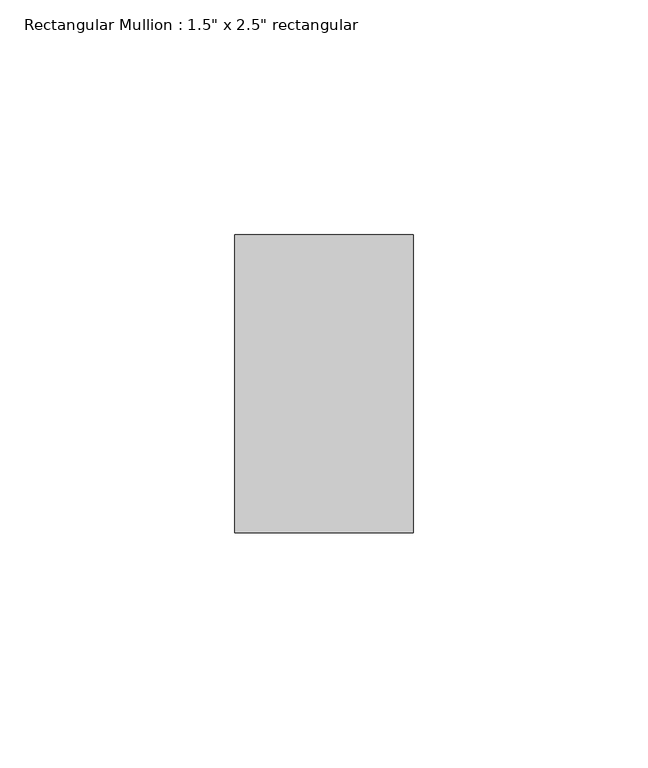
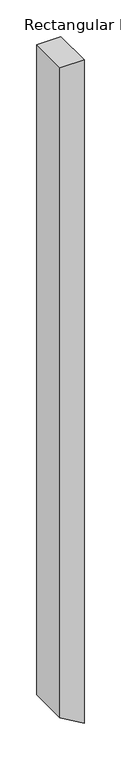
"""IFC4 building model written with IfcOpenShell, lengths in millimetres: member geometry."""

from ifc_helpers import new_model, si_unit, frame, origin, place, context, project, spatial, polyline, outline, extrude, source, transform, mapped, element, save


def member_ff75f20c(model_context):
    return source(origin(), model_context, "Body", "SweptSolid", [
        extrude(outline(polyline([(0.0, 19.05), (0.0, -19.05), (-1081.6731736, -19.05), (-1104.3176875, 19.05), (0.0, 19.05)])), frame((0.0, -31.75, 0.0), z_axis=(0.0, 1.0, 0.0), x_axis=(0.0, 0.0, 1.0)), (0.0, 0.0, 1.0), 63.5),
    ])


if __name__ == "__main__":
    model = new_model("IFC4")
    model_context = context("Model", 3, world=origin())
    ifc_project = project(units=[si_unit("LENGTHUNIT", "METRE", prefix="MILLI")], contexts=[model_context])
    site = spatial("IfcSite", under=ifc_project)
    building = spatial("IfcBuilding", under=site)
    placement = place(None, origin())
    member_shape = member_ff75f20c(model_context)
    element("IfcMember", 1, ObjectType="Rectangular Mullion : 1.5\" x 2.5\" rectangular", at=placement, inside=building, context=model_context, shape_type="MappedRepresentation", body=[
        mapped(member_shape, transform((0.0, 0.0, 0.0), x_axis=(1.0, 0.0, 0.0), y_axis=(0.0, 1.0, 0.0), z_axis=(0.0, 0.0, 1.0))),
    ])
    save(model, "model.ifc")

# Revit data of these elements
# Type "Rectangular Mullion : 1.5\" x 2.5\" rectangular"
#   built-in parameter 1007304 = 0.208333 (stored number, unit not read)
#   built-in parameter 1007301 = 0.0625 (stored number, unit not read)
#   built-in parameter 1007300 = 0.0625 (stored number, unit not read)
